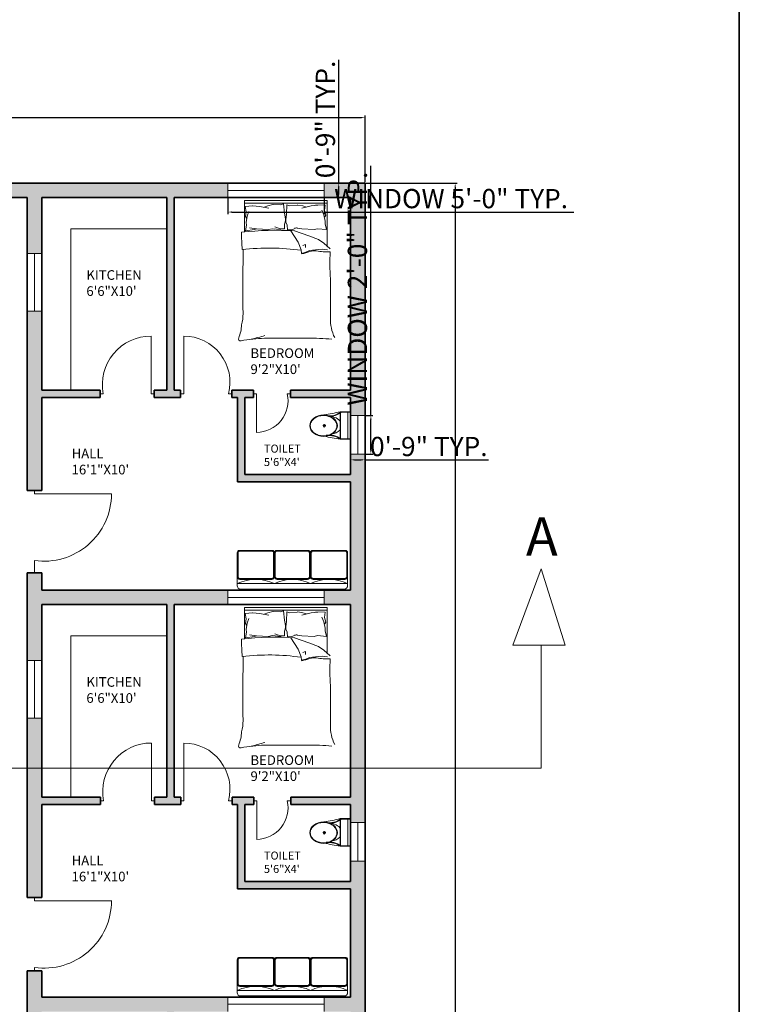
# Model space of a CAD drawing. Units: inches. Extents: x 1266 to 2869, y -408 to 3241.
# Tile 9 of 11: x 2420 to 2869, y 1767 to 2380. Entities that reach past the tile are written whole.
import ezdxf

# ---------------------------------------------------------------- set-up
doc = ezdxf.new("R2010")
doc.units = ezdxf.units.IN
for name, color, linetype, lineweight in [('A-ANNO-DIMS', 2, 'Continuous', 18), ('A-ANNO-SYMB', 7, 'Continuous', 18), ('A-ANNO-TTLB', 7, 'Continuous', 35), ('A-AREA-IDEN', 7, 'Continuous', 18), ('A-DOOR', 4, 'Continuous', 18), ('A-FLOR-CASE', 9, 'Continuous', 18), ('A-FLOR-FIXT', 9, 'Continuous', 18), ('A-FURN', 8, 'Continuous', 18), ('A-GLAZ', 4, 'Continuous', 18), ('A-WALL', 7, 'Continuous', 35), ('A-WALL-PATT', 251, 'Continuous', 13)]:
    doc.layers.add(name, color=color, linetype=linetype, lineweight=lineweight)
doc.styles.get("Standard").update_dxf_attribs({"font": 'arial.ttf'})
doc.dimstyles.new('ISO-25', dxfattribs={"dimtxt": 12, "dimasz": 2.5, "dimexe": 1.25, "dimexo": 0.625, "dimtad": 1, "dimdec": 0, "dimlunit": 3, "dimtxsty": 'Standard', "dimcen": 2.5, "dimadec": 0, "dimazin": 0, "dimtfac": 1, "dimtdec": 0, "dimtmove": 0, "dimatfit": 3, "dimfxl": 1, "dimarcsym": 0})

# ---------------------------------------------------------------- blocks, each defined once
blk = doc.blocks.new('A$C31115884')
for p, q in [((283, 498), (223, 498)), ((258, 466), (258, 523)), ((0, 200), (0, 0)), ((520, 200), (0, 200)), ((10, 190), (10, 10)), ((510, 190), (10, 190)), ((510, 10), (510, 190)), ((520, 0), (520, 200)), ((510, 54), (0, 54)), ((10, 10), (510, 10)), ((0, 0), (520, 0))]:
    blk.add_line(p, q)
blk.add_circle((256, 496), 23.6)
for centre, radius, start, end in [((2778, -205), 2807, 165.4549, 171.7133), ((-295, 403), 365, 324.2091, 9.3499), ((-295, 403), 375, 324.2091, 9.3499), ((139, 406), 293, 315.8436, 2.6563), ((806, 403), 375, 179.2036, 215.7909), ((806, 403), 365, 170.6501, 215.7909), ((3237, 905), 2807, 188.2867, 194.5451), ((384, 406), 293, 190.2774, 224.1564)]:
    blk.add_arc(centre, radius, start, end)
blk.add_ellipse((256, 510), major_axis=(0, -261), ratio=0.772727)
blk.add_open_spline([(256, 259), (263, 259), (270, 260), (288, 262), (299, 265), (320, 273), (330, 278), (350, 291), (360, 299), (378, 316), (386, 326), (402, 347), (409, 358), (421, 383), (427, 395), (436, 422), (440, 436), (445, 465), (447, 480), (448, 509), (448, 524), (445, 553), (443, 568), (436, 596), (432, 610), (422, 636), (416, 649), (402, 672), (395, 683), (379, 703), (370, 712), (351, 728), (341, 735), (321, 746), (310, 751), (289, 757), (278, 759), (256, 761), (245, 761), (223, 757), (212, 754), (191, 746), (181, 741), (161, 728), (151, 720), (133, 703), (125, 693), (110, 672), (103, 660), (90, 636), (85, 623), (76, 596), (72, 582), (67, 553), (66, 538), (64, 509), (65, 494), (68, 465), (70, 450), (77, 422), (81, 408), (91, 382), (97, 370), (111, 346), (118, 335), (135, 316), (144, 307), (162, 291), (172, 284), (193, 273), (203, 269), (225, 262), (236, 260), (250, 259), (253, 259), (256, 259)], degree=3, knots=[0, 0, 0, 0, 0.110105, 0.110105, 0.285049, 0.285049, 0.459994, 0.459994, 0.634938, 0.634938, 0.809882, 0.809882, 0.984827, 0.984827, 1.159771, 1.159771, 1.334715, 1.334715, 1.50966, 1.50966, 1.684604, 1.684604, 1.859549, 1.859549, 2.034493, 2.034493, 2.209437, 2.209437, 2.384382, 2.384382, 2.559326, 2.559326, 2.73427, 2.73427, 2.909215, 2.909215, 3.084159, 3.084159, 3.259103, 3.259103, 3.434048, 3.434048, 3.608992, 3.608992, 3.783936, 3.783936, 3.958881, 3.958881, 4.133825, 4.133825, 4.30877, 4.30877, 4.483714, 4.483714, 4.658658, 4.658658, 4.833603, 4.833603, 5.008547, 5.008547, 5.183491, 5.183491, 5.358436, 5.358436, 5.53338, 5.53338, 5.708324, 5.708324, 5.883269, 5.883269, 6.058213, 6.058213, 6.233158, 6.233158, 6.283185, 6.283185, 6.283185, 6.283185])
blk = doc.blocks.new('*D4')
at = {"layer": 'A-ANNO-DIMS', "color": 0, "lineweight": -2, "transparency": 16777216}
for p, q in [((2152.45, 2278.97), (2152.45, 2320.42)), ((2154.95, 2319.17), (2632.95, 2319.17)), ((2635.45, 2278.97), (2635.45, 2320.42))]:
    blk.add_line(p, q, dxfattribs=at)
at = {"layer": 'A-ANNO-DIMS', "color": 0, "transparency": 16777216}
for points in [[(2154.95, 2319.59), (2154.95, 2318.76), (2152.45, 2319.17)], [(2632.95, 2319.59), (2632.95, 2318.76), (2635.45, 2319.17)]]:
    blk.add_solid(points, dxfattribs=at)
at = {"layer": 'Defpoints', "color": 0, "transparency": 16777216}
for p in [(2635.45, 2319.17), (2152.45, 2278.35), (2635.45, 2278.35)]:
    blk.add_point(p, dxfattribs=at)
at = {"layer": 'A-ANNO-DIMS', "color": 0, "transparency": 16777216, "insert": (2393.95, 2325.93), "char_height": 12, "attachment_point": 5}
blk.add_mtext('40\'-3"', dxfattribs=at)
blk = doc.blocks.new('*D5')
at = {"layer": 'A-ANNO-DIMS', "color": 0, "lineweight": -2, "transparency": 16777216}
for p, q in [((2636.08, 2278.35), (2692.86, 2278.35)), ((2691.61, 2275.85), (2691.61, 1179.85)), ((2636.08, 1177.35), (2692.86, 1177.35))]:
    blk.add_line(p, q, dxfattribs=at)
at = {"layer": 'A-ANNO-DIMS', "color": 0, "transparency": 16777216}
for points in [[(2691.19, 2275.85), (2692.02, 2275.85), (2691.61, 2278.35)], [(2691.19, 1179.85), (2692.02, 1179.85), (2691.61, 1177.35)]]:
    blk.add_solid(points, dxfattribs=at)
at = {"layer": 'Defpoints', "color": 0, "transparency": 16777216}
for p in [(2635.45, 2278.35), (2635.45, 1177.35), (2691.61, 1177.35)]:
    blk.add_point(p, dxfattribs=at)
at = {"layer": 'A-ANNO-DIMS', "color": 0, "transparency": 16777216, "insert": (2684.86, 1727.85), "char_height": 12, "attachment_point": 5, "rotation": 90}
blk.add_mtext('91\'-9"', dxfattribs=at)
blk = doc.blocks.new('BED-DOUBLE-2')
for p, q in [((3.76, 67.77), (3.76, 87.35)), ((3.76, 87.35), (55.42, 87.35)), ((55.42, 87.35), (55.42, 58.59)), ((3.76, 85.69), (55.42, 85.69)), ((4.21, 83.74), (8.84, 84.1)), ((4.21, 83.77), (4.84, 80.33)), ((4.84, 80.33), (4.37, 77.51)), ((5.46, 77.67), (6.55, 80.64)), ((8.84, 84.1), (8.96, 84.08)), ((8.96, 84.08), (13.09, 83.77)), ((13.09, 83.77), (19.03, 82.67)), ((16.06, 83.3), (18.25, 84.08)), ((18.25, 84.08), (21.37, 84.86)), ((21.37, 84.86), (21.72, 84.86)), ((21.72, 84.86), (26.53, 84.7)), ((26.53, 84.7), (28.09, 85.33)), ((28.09, 85.33), (28.71, 79.55)), ((30.24, 84.66), (29.98, 78.85)), ((31.84, 84.13), (30.24, 84.66)), ((36.63, 84.59), (31.84, 84.13)), ((36.98, 84.61), (36.63, 84.59)), ((40.14, 84.02), (36.98, 84.61)), ((45.31, 84.03), (39.45, 82.57)), ((42.38, 83.38), (40.14, 84.02)), ((49.42, 84.6), (45.31, 84.03)), ((54.17, 84.59), (48.33, 84.69)), ((48.33, 84.69), (49.42, 84.6)), ((53.31, 78.43), (52.03, 81.32)), ((54.17, 84.59), (53.76, 81.12)), ((53.76, 81.12), (54.41, 78.34)), ((4.37, 77.51), (4.99, 76.42)), ((4.84, 73.76), (5.46, 77.67)), ((5.15, 72.04), (4.84, 73.76)), ((28.71, 79.55), (29.34, 76.11)), ((29.34, 74.7), (28.71, 72.67)), ((29.34, 76.11), (29.34, 74.7)), ((29.98, 78.85), (29.57, 75.38)), ((29.57, 75.38), (29.66, 73.97)), ((29.66, 73.97), (30.41, 71.98)), ((54.17, 74.56), (53.31, 78.43)), ((54.41, 78.34), (53.85, 77.21)), ((53.97, 72.83), (54.17, 74.56)), ((4.52, 68.61), (5.15, 72.04)), ((10.03, 69.39), (4.52, 68.61)), ((6.9, 70.46), (11.26, 69.74)), ((11.26, 69.74), (10.03, 69.39)), ((11.26, 69.74), (18.84, 69.27)), ((18.84, 69.27), (20.95, 69.87)), ((20.95, 69.87), (26.5, 69.44)), ((26.06, 69.77), (22.66, 70.95)), ((28.71, 69.77), (26.06, 69.77)), ((28.71, 72.67), (28.71, 69.77)), ((30.41, 71.98), (30.59, 69.09)), ((30.59, 69.09), (33.24, 69.26)), ((32.71, 68.56), (37.24, 61.54)), ((33.24, 69.26), (36.56, 70.64)), ((43.94, 65.39), (34.92, 68.56)), ((35.2, 70.46), (39.56, 69.74)), ((39.56, 69.74), (47.14, 69.27)), ((47.14, 69.27), (49.26, 69.87)), ((49.26, 69.87), (54.81, 69.44)), ((54.81, 69.44), (53.97, 72.83)), ((37.24, 61.54), (39.08, 56.69)), ((49.96, 63.21), (43.94, 65.39)), ((53.15, 60.87), (49.96, 63.21)), ((39.08, 56.69), (39.42, 54.51)), ((40.12, 59.32), (41.78, 59.99)), ((41.87, 58.1), (41.78, 59.99, 4.18)), ((42.1, 55.18), (44.27, 56.19)), ((44.27, 56.19), (47.96, 56.69)), ((47.96, 56.69), (52.14, 57.02)), ((52.14, 57.02), (55.49, 56.69)), ((57.15, 57.36), (53.15, 60.87)), ((39.42, 54.51), (42.1, 55.18)), ((16.28, 1.69), (42.89, 1.69))]:
    blk.add_line(p, q)
for centre, radius, start, end in [((92.06, 65.63), 90.06, 178.72178, 185.60397), ((23.09, -109.45), 178.34, 86.08655, 96.78213), ((19.19, -81.63), 139.47, 81.78449, 96.90062), ((-180.86, 53.65), 183.89, 358.4762, 1.00819), ((33.68, 85.75), 32.06, 280.66171, 289.88058), ((47.29, 49.44), 6.73, 78.6608, 113.73842), ((55.49, 94.55), 39.11, 259.87628, 272.56571), ((197.03, 48.09), 139.99, 176.97912, 183.83645), ((39.61, 54.45), 0.199, 160.24637, 271.13765), ((524.11, 32.64), 521.39, 178.22771, 181.71854), ((-4874.07, 14.03), 4931.49, 0.00217, 0.28689), ((-29.08, 17.61), 32.04, 346.06484, 358.91125), ((82.33, 13.12), 24.93, 177.47136, 206.46809), ((-23.41, 11.38), 25.47, 337.97508, 356.652), ((1.18, 1.17), 1.18, 146.17358, 293.47814), ((23.16, -129.76), 131.62, 92.99578, 99.40907), ((-18.62, 112.98), 115.08, 283.38322, 287.70533), ((44.49, -142.12), 143.82, 84.4998, 90.63509)]:
    blk.add_arc(centre, radius, start, end)
blk = doc.blocks.new('SOFA-3-SEAT')
for points in [[(0, 22.36), (0, 7.74, 0.414214), (1.72, 6.02), (21.5, 6.02, 0.414214), (23.22, 7.74), (23.22, 22.36, 0.414214), (21.5, 24.08), (1.72, 24.08, 0.414214)], [(0.52, 22.36), (0.52, 7.74, 0.414214), (1.72, 6.54), (21.5, 6.54, 0.414214), (22.7, 7.74), (22.7, 22.36, 0.414214), (21.5, 23.56), (1.72, 23.56, 0.414214)], [(45.57, 22.36), (45.57, 7.74, -0.414214), (43.85, 6.02), (24.94, 6.02, -0.414214), (23.22, 7.74), (23.22, 22.36, -0.414214), (24.94, 24.08), (43.85, 24.08, -0.414214)], [(45.06, 22.36), (45.06, 7.74, -0.414214), (43.85, 6.54), (24.94, 6.54, -0.414214), (23.73, 7.74), (23.73, 22.36, -0.414214), (24.94, 23.56), (43.85, 23.56, -0.414214)], [(45.57, 22.36), (45.57, 7.74, 0.414214), (47.29, 6.02), (67.07, 6.02, 0.414214), (68.79, 7.74), (68.79, 22.36, 0.414214), (67.07, 24.08), (47.29, 24.08, 0.414214)], [(46.09, 22.36), (46.09, 7.74, 0.414214), (47.29, 6.54), (67.07, 6.54, 0.414214), (68.27, 7.74), (68.27, 22.36, 0.414214), (67.07, 23.56), (47.29, 23.56, 0.414214)]]:
    blk.add_lwpolyline(points, format="xyb", close=True)
at = {"ltscale": 0.03}
blk.add_lwpolyline([(21.82, 24.08), (1.38, 24.08, 0.414214), (0, 22.7), (0, 2.06, 0.414214), (2.06, 0), (66.73, 0, 0.414214), (68.79, 2.06), (68.79, 22.7, 0.414214), (67.41, 24.08), (46.97, 24.08, 0.414214), (45.59, 22.7, -1), (45.56, 22.7, 0.414214), (44.18, 24.08), (24.61, 24.08, 0.414214), (23.23, 22.7, -1), (23.2, 22.7, 0.414214)], format="xyb", close=True, dxfattribs=at)
blk.add_lwpolyline([(0, 3.44), (68.79, 3.44)])
for centre, radius, start, end in [((11.61, -21.35), 27.38, 64.91063, 115.08937), ((34.4, -19.35), 25.38, 63.869, 116.131), ((57.18, -21.07), 27.12, 64.65382, 115.34618)]:
    blk.add_arc(centre, radius, start, end)
blk = doc.blocks.new('DOOR-KITCHEN-R')
for p, q in [((31.78, 0), (31.78, 36)), ((0, 0), (2, 0)), ((33.78, 0), (31.78, 0))]:
    blk.add_line(p, q)
blk.add_arc((31.78, 5.68), 30.32, 90, 190.7956)
blk = doc.blocks.new('DOOR-BEDROOM-R')
for p, q in [((2, 0), (2, 36)), ((0, 0), (2, 0)), ((31.84, 0), (29.84, 0))]:
    blk.add_line(p, q)
blk.add_arc((2, 7.24), 28.76, 345.43182, 90)
blk = doc.blocks.new('DOOR-BATH-R')
for p, q in [((0, 24), (2, 24)), ((2, 24), (2, 0)), ((23.14, 24), (21.14, 24))]:
    blk.add_line(p, q)
blk.add_arc((2, 19.63), 19.63, 270, 12.84994)
blk = doc.blocks.new('DOOR-ENTRY-R')
for p, q in [((0, 51.27), (0, 49.27)), ((0, 49.27), (36, 49.27)), ((36, 49.27), (48, 49.27)), ((0, 5.68), (0, 7.68)), ((0, 0), (0, 5.68))]:
    blk.add_line(p, q)
blk.add_arc((5.98, 49.27), 42.02, 261.81164, 0)
blk = doc.blocks.new('WIN-PLAN-60')
for p, q in [((0, 9), (0, 0)), ((60, 4.5), (60, 9)), ((60, 9), (60, 0)), ((0, 4.5), (60, 4.5)), ((0, 0), (0, 4.5))]:
    blk.add_line(p, q)
blk = doc.blocks.new('WIN-PLAN-36')
for p, q in [((0, 36), (9, 36)), ((4.5, 36), (4.5, 0)), ((9, 36), (4.5, 36)), ((4.5, 0), (0, 0)), ((0, 0), (9, 0))]:
    blk.add_line(p, q)
blk = doc.blocks.new('WIN-PLAN-24')
for p, q in [((0, 24), (9, 24)), ((4.5, 24), (4.5, 0)), ((9, 24), (4.5, 24)), ((0, 0), (9, 0))]:
    blk.add_line(p, q)
blk = doc.blocks.new('WIN-PLAN-24-2')
for p, q in [((0, 24), (9, 24)), ((4.5, 24), (4.5, 0)), ((9, 24), (4.5, 24)), ((4.5, 0), (0, 0)), ((0, 0), (9, 0))]:
    blk.add_line(p, q)
blk = doc.blocks.new('COUNTER-KITCHEN')
for p, q in [((0, 0), (0, 100.54)), ((0, 100.54), (59.82, 100.54))]:
    blk.add_line(p, q)
blk = doc.blocks.new('*D37')
at = {"layer": 'A-ANNO-DIMS', "color": 0, "lineweight": -2, "transparency": 16777216}
for p, q in [((2550.01, 2268.72), (2550.01, 2259.1)), ((2610.01, 2268.72), (2610.01, 2259.1)), ((2552.51, 2260.35), (2607.51, 2260.35)), ((2610.01, 2260.35), (2765.61, 2260.35))]:
    blk.add_line(p, q, dxfattribs=at)
at = {"layer": 'A-ANNO-DIMS', "color": 0, "transparency": 16777216}
for points in [[(2552.51, 2260.76), (2552.51, 2259.93), (2550.01, 2260.35)], [(2607.51, 2260.76), (2607.51, 2259.93), (2610.01, 2260.35)]]:
    blk.add_solid(points, dxfattribs=at)
at = {"layer": 'Defpoints', "color": 0, "transparency": 16777216}
for p in [(2550.01, 2269.35), (2610.01, 2269.35), (2610.01, 2260.35)]:
    blk.add_point(p, dxfattribs=at)
at = {"layer": 'A-ANNO-DIMS', "color": 0, "transparency": 16777216, "insert": (2689.06, 2267.18), "char_height": 12, "attachment_point": 5}
blk.add_mtext('WINDOW 5\'-0" TYP.', dxfattribs=at)
blk = doc.blocks.new('*D38')
at = {"layer": 'A-ANNO-DIMS', "color": 0, "lineweight": -2, "transparency": 16777216}
for p, q in [((2619.01, 2278.35), (2619.01, 2355.24)), ((2610.64, 2278.35), (2620.26, 2278.35)), ((2619.01, 2271.85), (2619.01, 2275.85)), ((2610.64, 2269.35), (2620.26, 2269.35))]:
    blk.add_line(p, q, dxfattribs=at)
at = {"layer": 'A-ANNO-DIMS', "color": 0, "transparency": 16777216}
for points in [[(2618.6, 2275.85), (2619.43, 2275.85), (2619.01, 2278.35)], [(2618.6, 2271.85), (2619.43, 2271.85), (2619.01, 2269.35)]]:
    blk.add_solid(points, dxfattribs=at)
at = {"layer": 'Defpoints', "color": 0, "transparency": 16777216}
for p in [(2610.01, 2278.35), (2619.01, 2278.35), (2610.01, 2269.35)]:
    blk.add_point(p, dxfattribs=at)
at = {"layer": 'A-ANNO-DIMS', "color": 0, "transparency": 16777216, "insert": (2612.26, 2318.05), "char_height": 12, "attachment_point": 5, "rotation": 90}
blk.add_mtext('0\'-9" TYP.', dxfattribs=at)
blk = doc.blocks.new('*D65')
at = {"layer": 'A-ANNO-DIMS', "color": 0, "lineweight": -2, "transparency": 16777216}
for p, q in [((2639.05, 2133.61), (2639.05, 2289.21)), ((2636.08, 2133.61), (2640.3, 2133.61)), ((2639.05, 2112.11), (2639.05, 2131.11)), ((2636.08, 2109.61), (2640.3, 2109.61))]:
    blk.add_line(p, q, dxfattribs=at)
at = {"layer": 'A-ANNO-DIMS', "color": 0, "transparency": 16777216}
for points in [[(2638.63, 2131.11), (2639.47, 2131.11), (2639.05, 2133.61)], [(2638.63, 2112.11), (2639.47, 2112.11), (2639.05, 2109.61)]]:
    blk.add_solid(points, dxfattribs=at)
at = {"layer": 'Defpoints', "color": 0, "transparency": 16777216}
for p in [(2635.45, 2133.61), (2639.05, 2133.61), (2635.45, 2109.61)]:
    blk.add_point(p, dxfattribs=at)
at = {"layer": 'A-ANNO-DIMS', "color": 0, "transparency": 16777216, "insert": (2632.22, 2212.66), "char_height": 12, "attachment_point": 5, "rotation": 90}
blk.add_mtext('WINDOW 2\'-0" TYP.', dxfattribs=at)
blk = doc.blocks.new('*D66')
at = {"layer": 'A-ANNO-DIMS', "color": 0, "lineweight": -2, "transparency": 16777216}
for p, q in [((2626.45, 2108.98), (2626.45, 2104.76)), ((2628.95, 2106.01), (2632.95, 2106.01)), ((2635.45, 2108.98), (2635.45, 2104.76)), ((2635.45, 2106.01), (2712.35, 2106.01))]:
    blk.add_line(p, q, dxfattribs=at)
at = {"layer": 'A-ANNO-DIMS', "color": 0, "transparency": 16777216}
for points in [[(2628.95, 2106.43), (2628.95, 2105.59), (2626.45, 2106.01)], [(2632.95, 2106.43), (2632.95, 2105.59), (2635.45, 2106.01)]]:
    blk.add_solid(points, dxfattribs=at)
at = {"layer": 'Defpoints', "color": 0, "transparency": 16777216}
for p in [(2626.45, 2109.61), (2635.45, 2109.61), (2635.45, 2106.01)]:
    blk.add_point(p, dxfattribs=at)
at = {"layer": 'A-ANNO-DIMS', "color": 0, "transparency": 16777216, "insert": (2675.15, 2112.76), "char_height": 12, "attachment_point": 5}
blk.add_mtext('0\'-9" TYP.', dxfattribs=at)

msp = doc.modelspace()

# ---------------------------------------------------------------- hatches: boundary and pattern name
at = {"layer": 'A-WALL-PATT'}
h = msp.add_hatch(color=256, dxfattribs=at)
h.dxf.hatch_style = 1
h.paths.add_polyline_path([(2161.45, 2269.35), (2239.45, 2269.35), (2239.45, 2149.35), (2235.18, 2149.35), (2235.18, 2144.85), (2243.95, 2144.85), (2249.99, 2144.85), (2249.99, 2146.74), (2249.99, 2149.35), (2243.95, 2149.35), (2243.95, 2269.35), (2274.21, 2269.35), (2274.21, 2273.85), (2274.21, 2278.35), (2152.45, 2278.35), (2152.45, 2234.52), (2161.45, 2234.52)])
h.paths.add_polyline_path([(2550.01, 2278.35), (2424.95, 2278.35), (2372.95, 2278.35), (2334.21, 2278.35), (2334.21, 2269.35), (2363.95, 2269.35), (2363.95, 2149.35), (2328.7, 2149.35), (2328.7, 2144.85), (2363.95, 2144.85), (2363.95, 2133.61), (2372.95, 2133.61), (2372.95, 2269.35), (2424.95, 2269.35), (2424.95, 2234.52), (2433.95, 2234.52), (2433.95, 2269.35), (2511.95, 2269.35), (2511.95, 2149.35), (2504.09, 2149.35), (2504.09, 2144.85), (2520.49, 2144.85), (2520.49, 2149.35), (2516.45, 2149.35), (2516.45, 2269.35), (2550.01, 2269.35), (2550.01, 2273.85)])
h.paths.add_polyline_path([(2635.45, 2278.35), (2610.01, 2278.35), (2610.01, 2269.35), (2626.45, 2269.35), (2626.45, 2149.35), (2588.98, 2149.35), (2588.98, 2144.85), (2626.45, 2144.85), (2626.45, 2133.61), (2635.45, 2133.61)])
h.paths.add_polyline_path([(2560.45, 2144.85), (2565.84, 2144.85), (2565.84, 2149.35), (2552.33, 2149.35), (2552.33, 2144.85), (2555.95, 2144.85), (2555.95, 2092.35), (2626.45, 2092.35), (2626.45, 2086.89), (2626.45, 2024.85), (2610.01, 2024.85), (2610.01, 2015.85), (2626.45, 2015.85), (2626.45, 1895.85), (2589.21, 1895.85), (2589.21, 1891.35), (2626.45, 1891.35), (2626.45, 1880.11), (2635.45, 1880.11), (2635.45, 2086.89), (2635.45, 2109.61), (2626.45, 2109.61), (2626.45, 2096.85), (2560.45, 2096.85)])
h.paths.add_polyline_path([(2433.95, 2198.52), (2424.95, 2198.52), (2424.95, 2086.89), (2433.95, 2086.89), (2433.95, 2144.85), (2470.3, 2144.85), (2470.3, 2149.35), (2433.95, 2149.35)])
h.paths.add_polyline_path([(2372.95, 2109.61), (2363.95, 2109.61), (2363.95, 2096.85), (2297.95, 2096.85), (2297.95, 2144.85), (2304, 2144.85), (2304, 2149.35), (2293.45, 2149.35), (2287.11, 2149.35), (2287.11, 2144.85), (2293.45, 2144.85), (2293.45, 2092.35), (2363.95, 2092.35), (2363.95, 2086.89), (2372.95, 2086.89)], flags=17)
h.paths.add_polyline_path([(2161.45, 2144.85), (2197.56, 2144.85), (2197.56, 2149.35), (2161.45, 2149.35), (2161.45, 2198.52), (2152.45, 2198.52), (2152.45, 1981.02), (2161.45, 1981.02), (2161.45, 2015.85), (2363.95, 2015.85), (2363.95, 1895.85), (2326.89, 1895.85), (2326.89, 1891.35), (2363.95, 1891.35), (2363.95, 1880.11), (2372.95, 1880.11), (2372.95, 2035.62), (2363.95, 2035.62), (2363.95, 2024.85), (2161.45, 2024.85)])
h.paths.add_polyline_path([(2161.45, 1691.52), (2152.45, 1691.52), (2152.45, 1474.02), (2161.45, 1474.02)])
h.paths.add_polyline_path([(2194.79, 1895.85), (2161.45, 1895.85), (2161.45, 1945.02), (2152.45, 1945.02), (2152.45, 1727.52), (2161.45, 1727.52), (2161.45, 1762.35), (2363.95, 1762.35), (2363.95, 1642.35), (2328.7, 1642.35), (2328.7, 1637.85), (2363.95, 1637.85), (2363.95, 1589.85), (2297.95, 1589.85), (2297.95, 1637.85), (2303.95, 1637.85), (2303.95, 1642.35), (2287.64, 1642.35), (2287.64, 1637.85), (2293.45, 1637.85), (2293.45, 1585.35), (2363.95, 1585.35), (2363.95, 1579.45), (2372.95, 1579.45), (2372.95, 1779.84), (2363.95, 1779.84), (2363.95, 1771.35), (2161.45, 1771.35), (2161.45, 1891.35), (2194.79, 1891.35)])
h.paths.add_polyline_path([(2243.95, 2015.85), (2239.45, 2015.85), (2239.45, 1895.85), (2232.4, 1895.85), (2232.4, 1891.35), (2247.22, 1891.35), (2247.22, 1895.85), (2243.95, 1895.85)], flags=17)
h.paths.add_polyline_path([(2302.19, 1895.85), (2284.34, 1895.85), (2284.34, 1891.35), (2293.45, 1891.35), (2293.45, 1838.85), (2363.95, 1838.85), (2363.95, 1831.11), (2372.95, 1831.11), (2372.95, 1856.11), (2363.95, 1856.11), (2363.95, 1843.35), (2297.95, 1843.35), (2297.95, 1891.35), (2302.19, 1891.35)], flags=17)
h.paths.add_polyline_path([(2243.95, 1762.35), (2239.45, 1762.35), (2239.45, 1642.35), (2235.18, 1642.35), (2235.18, 1637.85), (2249.99, 1637.85), (2249.99, 1642.35), (2243.95, 1642.35)], flags=17)
h.paths.add_polyline_path([(2197.56, 1642.35), (2161.45, 1642.35), (2161.45, 1637.85), (2197.56, 1637.85)], flags=17)
h.paths.add_polyline_path([(2363.95, 1517.85), (2161.45, 1517.85), (2161.45, 1508.85), (2239.45, 1508.85), (2239.45, 1388.85), (2243.95, 1388.85), (2243.95, 1508.85), (2363.95, 1508.85)])
h.paths.add_polyline_path([(2372.95, 1528.18), (2363.95, 1528.18), (2363.95, 1323.21), (2372.95, 1323.21)])
h.paths.add_polyline_path([(2372.95, 1271.94), (2363.95, 1271.94), (2363.95, 1264.35), (2161.45, 1264.35), (2161.45, 1283.77), (2156.95, 1283.77), (2152.45, 1283.77), (2152.45, 1255.35), (2156.95, 1255.35), (2372.95, 1255.35)])
h.paths.add_polyline_path([(2161.45, 1438.02), (2152.45, 1438.02), (2152.45, 1319.77), (2161.45, 1319.77)])
h.paths.add_polyline_path([(2550.01, 1513.35), (2550.01, 1517.85), (2433.95, 1517.85), (2433.95, 1528.62), (2424.95, 1528.62), (2424.95, 1474.02), (2433.95, 1474.02), (2433.95, 1508.85), (2511.95, 1508.85), (2511.95, 1388.85), (2504.09, 1388.85), (2504.09, 1384.35), (2520.49, 1384.35), (2520.49, 1388.85), (2516.45, 1388.85), (2516.45, 1508.85), (2550.01, 1508.85)])
h.paths.add_polyline_path([(2635.45, 1602.61), (2626.45, 1602.61), (2626.45, 1517.85), (2610.01, 1517.85), (2610.01, 1508.85), (2626.45, 1508.85), (2626.45, 1388.85), (2588.98, 1388.85), (2588.98, 1384.35), (2626.45, 1384.35), (2626.45, 1373.11), (2635.45, 1373.11)])
h.paths.add_polyline_path([(2635.45, 1349.11), (2626.45, 1349.11), (2626.45, 1336.35), (2560.45, 1336.35), (2560.45, 1384.35), (2565.84, 1384.35), (2565.84, 1388.85), (2552.33, 1388.85), (2552.33, 1384.35), (2555.95, 1384.35), (2555.95, 1331.85), (2626.45, 1331.85), (2626.45, 1315.59), (2635.45, 1315.59)])
h.paths.add_polyline_path([(2635.45, 1279.59), (2630.95, 1279.59), (2626.45, 1279.59), (2626.45, 1264.35), (2433.95, 1264.35), (2433.95, 1275.12), (2424.95, 1275.12), (2424.95, 1255.35), (2635.45, 1255.35)])
h.paths.add_polyline_path([(2433.95, 1438.02), (2424.95, 1438.02), (2424.95, 1326.39), (2433.95, 1326.39)])
h.paths.add_polyline_path([(2470.3, 1388.85), (2433.95, 1388.85), (2433.95, 1384.35), (2470.3, 1384.35)], flags=0)
h = msp.add_hatch(color=256, dxfattribs=at)
h.dxf.hatch_style = 1
h.paths.add_polyline_path([(2550.01, 2020.35), (2550.01, 2024.85), (2433.95, 2024.85), (2433.95, 2035.62), (2424.95, 2035.62), (2424.95, 1981.02), (2433.95, 1981.02), (2433.95, 2015.85), (2511.95, 2015.85), (2511.95, 1895.85), (2504.33, 1895.85), (2504.33, 1891.35), (2520.72, 1891.35), (2520.72, 1895.85), (2516.45, 1895.85), (2516.45, 2015.85), (2550.01, 2015.85)])
h.paths.add_polyline_path([(2433.95, 1945.02), (2424.95, 1945.02), (2424.95, 1833.39), (2433.95, 1833.39), (2433.95, 1891.35), (2470.53, 1891.35), (2470.53, 1895.85), (2433.95, 1895.85)])
h.paths.add_polyline_path([(2550.01, 1771.35), (2433.95, 1771.35), (2433.95, 1787.8), (2424.95, 1787.8), (2424.95, 1727.52), (2433.95, 1727.52), (2433.95, 1762.35), (2511.95, 1762.35), (2511.95, 1642.35), (2504.09, 1642.35), (2504.09, 1637.85), (2520.49, 1637.85), (2520.49, 1642.35), (2516.45, 1642.35), (2516.45, 1762.35), (2550.01, 1762.35), (2550.01, 1766.85)])
h.paths.add_polyline_path([(2560.45, 1637.85), (2565.84, 1637.85), (2565.84, 1642.35), (2552.33, 1642.35), (2552.33, 1637.85), (2555.95, 1637.85), (2555.95, 1585.35), (2626.45, 1585.35), (2626.45, 1589.85), (2560.45, 1589.85)])
h.paths.add_polyline_path([(2635.45, 1856.11), (2626.45, 1856.11), (2626.45, 1843.35), (2560.45, 1843.35), (2560.45, 1891.35), (2566.07, 1891.35), (2566.07, 1895.85), (2552.56, 1895.85), (2552.56, 1891.35), (2555.95, 1891.35), (2555.95, 1838.85), (2626.45, 1838.85), (2626.45, 1771.35), (2610.01, 1771.35), (2610.01, 1762.35), (2626.45, 1762.35), (2626.45, 1642.35), (2588.98, 1642.35), (2588.98, 1637.85), (2626.45, 1637.85), (2626.45, 1626.61), (2635.45, 1626.61)])
h.paths.add_polyline_path([(2433.95, 1691.52), (2424.95, 1691.52), (2424.95, 1579.89), (2433.95, 1579.89)])
h.paths.add_polyline_path([(2470.3, 1642.35), (2433.95, 1642.35), (2433.95, 1637.85), (2470.3, 1637.85)], flags=17)

# ---------------------------------------------------------------- linework, layer by layer
at = {"layer": 'A-ANNO-SYMB'}
for p, q in [((2745.24, 2038.2), (2727.59, 1990.48)), ((2760.16, 1990.48), (2745.24, 2038.2)), ((2727.59, 1990.48), (2758.34, 1990.48)), ((2745.24, 1914.02), (2745.24, 1990.48)), ((2758.34, 1990.48), (2760.16, 1990.48)), ((2029.46, 1914.02), (2745.24, 1914.02))]:
    msp.add_line(p, q, dxfattribs=at)
at = {"layer": 'A-ANNO-TTLB'}
msp.add_lwpolyline([(1266.23, 3241.34), (2868.62, 3241.34), (2868.62, 986.84), (1266.23, 986.84)], close=True, dxfattribs=at)
at = {"layer": 'A-DOOR'}
for p, q in [((2522.49, 1893.6), (2522.49, 1929.6)), ((2470.53, 1893.6), (2472.3, 1893.6)), ((2504.09, 1893.6), (2502.32, 1893.6)), ((2520.72, 1893.6), (2522.49, 1893.6)), ((2520.72, 1893.6), (2522.49, 1893.6)), ((2552.33, 1893.6), (2550.33, 1893.6)), ((2552.56, 1893.6), (2550.56, 1893.6)), ((2566.07, 1893.6), (2568.07, 1893.6)), ((2568.07, 1893.6), (2568.07, 1869.6)), ((2588.98, 1893.6), (2586.98, 1893.6)), ((2589.21, 1893.6), (2587.21, 1893.6)), ((2429.45, 1833.39), (2429.45, 1831.39)), ((2429.45, 1831.39), (2465.45, 1831.39)), ((2429.68, 1831.39), (2465.68, 1831.39)), ((2465.45, 1831.39), (2477.45, 1831.39)), ((2465.68, 1831.39), (2477.68, 1831.39)), ((2429.45, 1787.8), (2429.45, 1789.8))]:
    msp.add_line(p, q, dxfattribs=at)
for centre, radius, start, end in [((2522.49, 1900.83), 28.76, 345.43182, 90), ((2567.84, 1889.23), 19.63, 270, 12.84994), ((2435.43, 1831.39), 42.02, 261.81164, 0)]:
    msp.add_arc(centre, radius, start, end, dxfattribs=at)
at = {"layer": 'A-FURN'}
for points in [[(2555.77, 1794.38), (2555.77, 1779.76, 0.414214), (2557.49, 1778.04), (2577.27, 1778.04, 0.414214), (2578.99, 1779.76), (2578.99, 1794.38, 0.414214), (2577.27, 1796.1), (2557.49, 1796.1, 0.414214)], [(2556.29, 1794.38), (2556.29, 1779.76, 0.414214), (2557.49, 1778.56), (2577.27, 1778.56, 0.414214), (2578.48, 1779.76), (2578.48, 1794.38, 0.414214), (2577.27, 1795.59), (2557.49, 1795.59, 0.414214)], [(2601.35, 1794.38), (2601.35, 1779.76, -0.414214), (2599.63, 1778.04), (2580.71, 1778.04, -0.414214), (2578.99, 1779.76), (2578.99, 1794.38, -0.414214), (2580.71, 1796.1), (2599.63, 1796.1, -0.414214)], [(2600.83, 1794.38), (2600.83, 1779.76, -0.414214), (2599.63, 1778.56), (2580.71, 1778.56, -0.414214), (2579.51, 1779.76), (2579.51, 1794.38, -0.414214), (2580.71, 1795.59), (2599.63, 1795.59, -0.414214)], [(2601.35, 1794.38), (2601.35, 1779.76, 0.414214), (2603.07, 1778.04), (2622.85, 1778.04, 0.414214), (2624.57, 1779.76), (2624.57, 1794.38, 0.414214), (2622.85, 1796.1), (2603.07, 1796.1, 0.414214)], [(2601.86, 1794.38), (2601.86, 1779.76, 0.414214), (2603.07, 1778.56), (2622.85, 1778.56, 0.414214), (2624.05, 1779.76), (2624.05, 1794.38, 0.414214), (2622.85, 1795.59), (2603.07, 1795.59, 0.414214)]]:
    msp.add_lwpolyline(points, format="xyb", close=True, dxfattribs=at)
at = {"layer": 'A-FURN', "ltscale": 0.03}
msp.add_lwpolyline([(2577.6, 1796.1), (2557.15, 1796.1, 0.414214), (2555.77, 1794.73), (2555.77, 1774.09, 0.414214), (2557.84, 1772.03), (2622.5, 1772.03, 0.414214), (2624.57, 1774.09), (2624.57, 1794.73, 0.414214), (2623.19, 1796.1), (2602.74, 1796.1, 0.414214), (2601.37, 1794.73, -1), (2601.33, 1794.73, 0.414214), (2599.96, 1796.1), (2580.38, 1796.1, 0.414214), (2579.01, 1794.73, -1), (2578.97, 1794.73, 0.414214)], format="xyb", close=True, dxfattribs=at)
at = {"layer": 'A-FURN'}
msp.add_lwpolyline([(2555.77, 1775.47), (2624.57, 1775.47)], dxfattribs=at)
for centre, radius, start, end in [((2567.38, 1750.67), 27.38, 64.91063, 115.08937), ((2590.17, 1752.68), 25.38, 63.869, 116.131), ((2612.96, 1750.96), 27.12, 64.65382, 115.34618)]:
    msp.add_arc(centre, radius, start, end, dxfattribs=at)
at = {"layer": 'A-WALL'}
for p, q in [((2372.95, 2278.35), (2424.95, 2278.35)), ((2424.95, 2278.35), (2635.45, 2278.35)), ((2635.45, 2278.35), (2635.45, 2086.89)), ((2424.95, 2269.35), (2372.95, 2269.35)), ((2424.95, 2269.35), (2424.95, 2086.89)), ((2433.95, 2269.35), (2433.95, 2149.35)), ((2433.95, 2269.35), (2511.95, 2269.35)), ((2511.95, 2269.35), (2511.95, 2149.35)), ((2516.45, 2269.35), (2516.45, 2149.35)), ((2516.45, 2269.35), (2626.45, 2269.35)), ((2626.45, 2269.35), (2626.45, 2149.35)), ((2433.95, 2149.35), (2470.3, 2149.35)), ((2470.3, 2149.35), (2470.3, 2144.85)), ((2504.09, 2149.35), (2511.95, 2149.35)), ((2504.09, 2149.35), (2504.09, 2144.85)), ((2516.45, 2149.35), (2520.49, 2149.35)), ((2520.49, 2149.35), (2520.49, 2144.85)), ((2520.49, 2149.35), (2520.49, 2144.85)), ((2552.33, 2149.35), (2565.84, 2149.35)), ((2552.33, 2149.35), (2552.33, 2144.85)), ((2565.84, 2149.35), (2565.84, 2144.85)), ((2588.98, 2149.35), (2626.45, 2149.35)), ((2588.98, 2149.35), (2588.98, 2144.85)), ((2433.95, 2144.85), (2433.95, 2086.89)), ((2433.95, 2144.85), (2470.3, 2144.85)), ((2504.09, 2144.85), (2520.49, 2144.85)), ((2552.33, 2144.85), (2555.95, 2144.85)), ((2555.95, 2144.85), (2555.95, 2092.35)), ((2560.45, 2144.85), (2560.45, 2096.85)), ((2560.45, 2144.85), (2565.84, 2144.85)), ((2588.98, 2144.85), (2626.45, 2144.85)), ((2626.45, 2144.85), (2626.45, 2096.85)), ((2555.95, 2092.35), (2626.45, 2092.35)), ((2560.45, 2096.85), (2626.45, 2096.85)), ((2626.45, 2092.35), (2626.45, 2086.89)), ((2424.95, 2086.89), (2433.95, 2086.89)), ((2626.45, 2086.89), (2626.45, 2024.85)), ((2635.45, 1255.35), (2635.45, 2086.89)), ((2424.95, 2035.62), (2424.95, 1833.39)), ((2424.95, 2035.62), (2433.95, 2035.62)), ((2433.95, 2035.62), (2433.95, 2024.85)), ((2433.95, 2024.85), (2626.45, 2024.85)), ((2433.95, 2015.85), (2433.95, 1895.85)), ((2433.95, 2015.85), (2511.95, 2015.85)), ((2511.95, 2015.85), (2511.95, 1895.85)), ((2516.45, 2015.85), (2516.45, 1895.85)), ((2516.45, 2015.85), (2626.45, 2015.85)), ((2626.45, 2015.85), (2626.45, 1895.85)), ((2433.95, 1895.85), (2470.53, 1895.85)), ((2470.53, 1893.6), (2470.53, 1895.85)), ((2470.53, 1895.85), (2470.53, 1891.35)), ((2504.33, 1895.85), (2511.95, 1895.85)), ((2504.33, 1891.35), (2504.33, 1895.85)), ((2516.45, 1895.85), (2520.72, 1895.85)), ((2520.72, 1891.35), (2520.72, 1895.85)), ((2552.56, 1895.85), (2566.07, 1895.85)), ((2552.56, 1891.35), (2552.56, 1895.85)), ((2566.07, 1891.35), (2566.07, 1895.85)), ((2589.21, 1895.85), (2626.45, 1895.85)), ((2589.21, 1891.35), (2589.21, 1895.85)), ((2433.95, 1891.35), (2433.95, 1833.39)), ((2433.95, 1891.35), (2470.53, 1891.35)), ((2504.33, 1891.35), (2520.72, 1891.35)), ((2520.72, 1893.6), (2520.72, 1891.35)), ((2552.56, 1893.6), (2552.56, 1891.35)), ((2552.56, 1891.35), (2555.95, 1891.35)), ((2555.95, 1891.35), (2555.95, 1838.85)), ((2560.45, 1891.35), (2566.07, 1891.35)), ((2560.45, 1891.35), (2560.45, 1843.35)), ((2589.21, 1893.6), (2589.21, 1891.35)), ((2589.21, 1891.35), (2626.45, 1891.35)), ((2589.21, 1891.35), (2589.21, 1891.35)), ((2626.45, 1891.35), (2626.45, 1843.35)), ((2560.45, 1843.35), (2626.45, 1843.35)), ((2555.95, 1838.85), (2626.45, 1838.85)), ((2626.45, 1838.85), (2626.45, 1771.35)), ((2429.68, 1833.39), (2424.95, 1833.39)), ((2424.95, 1833.39), (2433.95, 1833.39)), ((2424.95, 1787.8), (2424.95, 1579.89)), ((2433.95, 1787.8), (2424.95, 1787.8)), ((2429.68, 1787.8), (2433.95, 1787.8)), ((2433.95, 1787.8), (2433.95, 1771.35)), ((2433.95, 1771.35), (2626.45, 1771.35))]:
    msp.add_line(p, q, dxfattribs=at)

# ---------------------------------------------------------------- block references
at = {"layer": 'A-DOOR'}
for name, p in [('DOOR-KITCHEN-R', (2470.3, 2147.1)), ('DOOR-BEDROOM-R', (2520.49, 2147.1)), ('DOOR-BATH-R', (2565.84, 2123.1)), ('DOOR-ENTRY-R', (2429.45, 2035.62)), ('DOOR-KITCHEN-R', (2470.53, 1893.6))]:
    msp.add_blockref(name, p, dxfattribs=at)
at = {"layer": 'A-FLOR-CASE'}
for p in [(2452.13, 2149.35), (2452.13, 1895.85)]:
    msp.add_blockref('COUNTER-KITCHEN', p, dxfattribs=at)
at = {"layer": 'A-FLOR-FIXT', "xscale": 0.0330640103915726, "yscale": 0.0330640103915726, "zscale": 0.0330640103915726, "rotation": 89.99999999999996}
for p in [(2626.45, 2118.81), (2626.45, 1865.31)]:
    msp.add_blockref('A$C31115884', p, dxfattribs=at)
at = {"layer": 'A-FURN'}
for name, p in [('BED-DOUBLE-2', (2556.51, 2180.11)), ('SOFA-3-SEAT', (2555.77, 2025.53)), ('BED-DOUBLE-2', (2556.51, 1926.61))]:
    msp.add_blockref(name, p, dxfattribs=at)
at = {"layer": 'A-GLAZ'}
for name, p in [('WIN-PLAN-60', (2550.01, 2269.35)), ('WIN-PLAN-36', (2424.95, 2198.52)), ('WIN-PLAN-24-2', (2626.45, 2109.61)), ('WIN-PLAN-60', (2550.01, 2015.85)), ('WIN-PLAN-36', (2424.95, 1945.02)), ('WIN-PLAN-24', (2626.45, 1856.11)), ('WIN-PLAN-60', (2550.01, 1762.35))]:
    msp.add_blockref(name, p, dxfattribs=at)

# ---------------------------------------------------------------- texts
at = {"layer": 'A-ANNO-SYMB', "insert": (2735.63, 2070.22), "char_height": 24, "attachment_point": 1}
msp.add_mtext_dynamic_manual_height_columns('A', width=125.6117, gutter_width=12.5, heights=[0], dxfattribs=at)
at = {"layer": 'A-AREA-IDEN', "attachment_point": 1}
for s, width, insert, char_height in [('KITCHEN\\P6\'6"X10\'', 112.1355, (2461.8, 2224.14), 6), ('BEDROOM\\P9\'2"X10\'', 62.026, (2564.06, 2175.46), 6), ('HALL\\P16\'1"X10\'', 100.9767, (2452.62, 2112.93), 6), ('TOILET\\P5\'6"X4\'', 46.3569, (2572.45, 2115.49), 5), ('KITCHEN\\P6\'6"X10\'', 112.1355, (2461.8, 1970.64), 6), ('BEDROOM\\P9\'2"X10\'', 62.026, (2564.06, 1921.96), 6), ('HALL\\P16\'1"X10\'', 100.9767, (2452.62, 1859.43), 6), ('TOILET\\P5\'6"X4\'', 46.3569, (2572.45, 1861.99), 5)]:
    msp.add_mtext_dynamic_manual_height_columns(s, width=width, gutter_width=12.5, heights=[0], dxfattribs=dict(at, insert=insert, char_height=char_height))

# ---------------------------------------------------------------- dimensions: what is measured, and where the dimension line sits
at = {"layer": 'A-ANNO-DIMS'}
for base, p1, p2, text, picture, middle in [((2619.01, 2278.35), (2610.01, 2269.35), (2610.01, 2278.35), '<> TYP.', '*D38', (2612.26, 2318.05)), ((2639.05, 2133.61), (2635.45, 2109.61), (2635.45, 2133.61), 'WINDOW <> TYP.', '*D65', (2632.22, 2212.66))]:
    dim = msp.add_linear_dim(base=base, p1=p1, p2=p2, angle=90, text=text, dimstyle='ISO-25', override={"dimdec": 1, "dimlfac": 1, "dimrnd": 0, "dimzin": 1, "dimdsep": 46, "dimlunit": 4, "dimfrac": 2}, dxfattribs=at)
    dim.commit()
    dim.dimension.update_dxf_attribs({"geometry": picture, "text_midpoint": middle})
dim = msp.add_linear_dim(base=(2635.45, 2319.17), p1=(2152.45, 2278.35), p2=(2635.45, 2278.35), dimstyle='ISO-25', override={"dimclrd": 0, "dimclre": 0, "dimclrt": 0}, dxfattribs=at)
dim.commit()
dim.dimension.update_dxf_attribs({"geometry": '*D4', "text_midpoint": (2393.95, 2319.17), "dimtype": 160})
for base, p1, p2, text, picture, middle in [((2610.01, 2260.35), (2550.01, 2269.35), (2610.01, 2269.35), 'WINDOW <> TYP.', '*D37', (2689.06, 2267.18)), ((2635.45, 2106.01), (2626.45, 2109.61), (2635.45, 2109.61), '<> TYP.', '*D66', (2675.15, 2112.76))]:
    dim = msp.add_linear_dim(base=base, p1=p1, p2=p2, text=text, dimstyle='ISO-25', override={"dimdec": 1, "dimlfac": 1, "dimrnd": 0, "dimzin": 1, "dimdsep": 46, "dimlunit": 4, "dimfrac": 2}, dxfattribs=at)
    dim.commit()
    dim.dimension.update_dxf_attribs({"geometry": picture, "text_midpoint": middle})
dim = msp.add_linear_dim(base=(2691.61, 1177.35), p1=(2635.45, 2278.35), p2=(2635.45, 1177.35), angle=90, dimstyle='ISO-25', override={"dimclrd": 0, "dimclre": 0, "dimclrt": 0}, dxfattribs=at)
dim.commit()
dim.dimension.update_dxf_attribs({"geometry": '*D5', "text_midpoint": (2684.86, 1727.85)})

doc.saveas('drawing.dxf')
